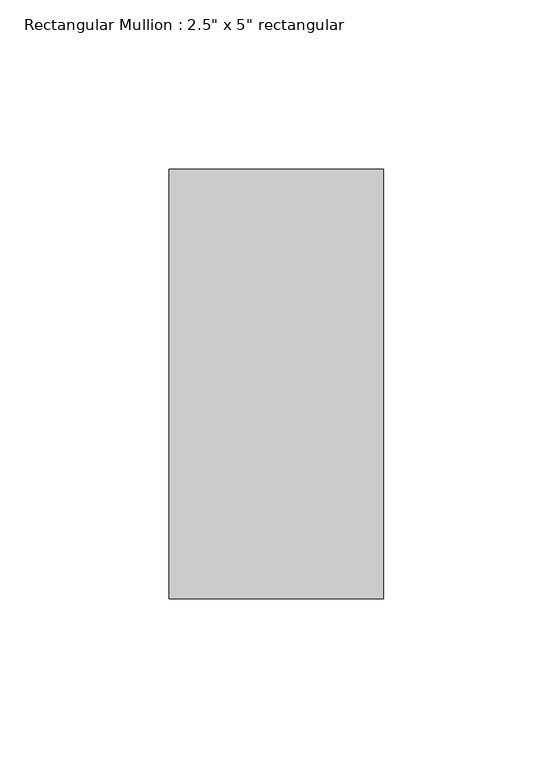
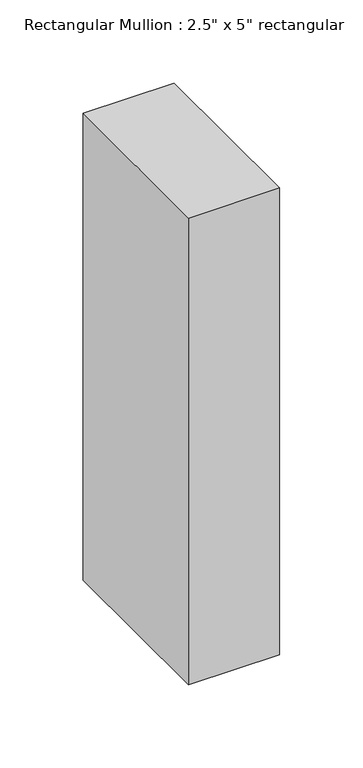
"""IFC4 building model written with IfcOpenShell, lengths in millimetres: member geometry."""

from ifc_helpers import new_model, si_unit, frame, origin, place, context, project, spatial, polyline, outline, extrude, source, transform, mapped, element, save


def member_ff1b7d8f(model_context):
    return source(origin(), model_context, "Body", "SweptSolid", [
        extrude(outline(polyline([(0.0, 63.5), (0.0, -63.5), (-63.5, -63.5), (-63.5, 63.5), (0.0, 63.5)])), frame((0.0, 0.0, -342.9), z_axis=(0.0, 0.0, 1.0), x_axis=(1.0, 0.0, 0.0)), (0.0, 0.0, 1.0), 342.9),
    ])


if __name__ == "__main__":
    model = new_model("IFC4")
    model_context = context("Model", 3, world=origin())
    ifc_project = project(units=[si_unit("LENGTHUNIT", "METRE", prefix="MILLI")], contexts=[model_context])
    site = spatial("IfcSite", under=ifc_project)
    building = spatial("IfcBuilding", under=site)
    placement = place(None, origin())
    member_shape = member_ff1b7d8f(model_context)
    element("IfcMember", 1, ObjectType="Rectangular Mullion : 2.5\" x 5\" rectangular", at=placement, inside=building, context=model_context, shape_type="MappedRepresentation", body=[
        mapped(member_shape, transform((0.0, 0.0, 0.0), x_axis=(1.0, 0.0, 0.0), y_axis=(0.0, 1.0, 0.0), z_axis=(0.0, 0.0, 1.0))),
    ])
    save(model, "model.ifc")

# Revit data of these elements
# Type "Rectangular Mullion : 2.5\" x 5\" rectangular"
#   built-in parameter 1007304 = 0.416667 (stored number, unit not read)
#   built-in parameter 1007301 = 0.104167 (stored number, unit not read)
#   built-in parameter 1007300 = 0.104167 (stored number, unit not read)
